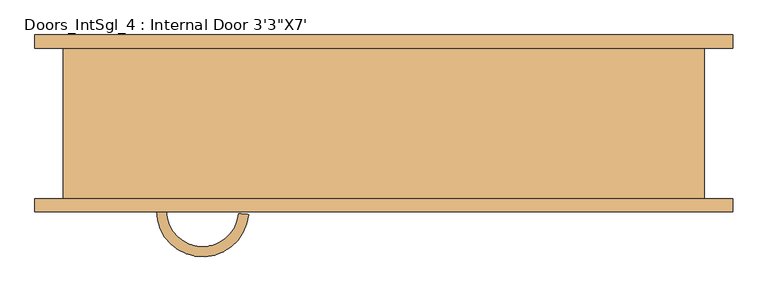
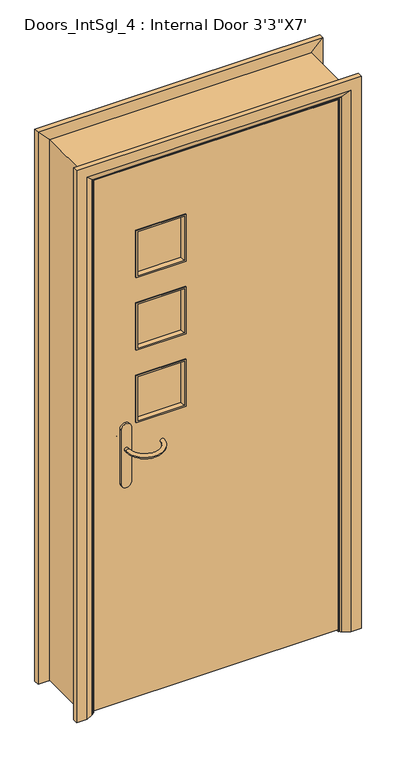
"""IFC4 building model written with IfcOpenShell, lengths in millimetres: door geometry."""

from ifc_helpers import new_model, si_unit, point, frame, frame_2d, origin, place, context, project, spatial, polyline, circle_curve, ellipse_curve, trimmed, segment, composite_curve, outline, extrude, faceted_brep, source, transform, mapped, element, save
from ifc_brep_helpers import plane_surface, cylinder_surface, revolved_surface, advanced_brep


def door_cca51ba5(model_context):
    return source(origin(), model_context, "Body", "SolidModel", [
        advanced_brep(
        [(-345.5, -68.3, 1000.0), (-330.5, -68.3, 1000.0), (-345.5, -58.3, 1000.0), (-330.5, -58.3, 1000.0), (-205.5986682, -52.1917759, 1000.0), (-220.5415886, -53.4991121, 1000.0)],
        [
            (0, 1, circle_curve(frame((-338.0, -68.3, 1000.0), z_axis=(0.0, -1.0, 0.0), x_axis=(1.0, 0.0, 0.0)), 7.5)),
            (1, 0, circle_curve(frame((-338.0, -68.3, 1000.0), z_axis=(0.0, -1.0, 0.0), x_axis=(1.0, 0.0, 0.0)), 7.5)),
            (0, 2),
            (2, 3, circle_curve(frame((-338.0, -58.3, 1000.0), z_axis=(0.0, -1.0, 0.0), x_axis=(1.0, 0.0, 0.0)), 7.5)),
            (3, 1),
            (3, 2, circle_curve(frame((-338.0, -58.3, 1000.0), z_axis=(0.0, -1.0, 0.0), x_axis=(1.0, 0.0, 0.0)), 7.5)),
            (4, 5, circle_curve(frame((-213.0701284, -52.845444, 1000.0), z_axis=(0.08715574274766678, -0.9961946980917448, 0.0), x_axis=(-0.9961946980917448, -0.08715574274766678, 0.0)), 7.5)),
            (5, 4, circle_curve(frame((-213.0701284, -52.845444, 1000.0), z_axis=(0.08715574274766678, -0.9961946980917448, 0.0), x_axis=(-0.9961946980917448, -0.08715574274766678, 0.0)), 7.5)),
            (5, 3, circle_curve(frame((-275.4159887, -58.3, 1000.0), z_axis=(0.0, 0.0, 1.0), x_axis=(-1.0, 0.0, 0.0)), 55.0840113)),
            (2, 4, circle_curve(frame((-275.4159887, -58.3, 1000.0), z_axis=(0.0, 0.0, -1.0), x_axis=(-1.0, 0.0, 0.0)), 70.0840113)),
        ],
        [
            plane_surface(frame((-338.0, -68.3, 1000.0), z_axis=(0.0, -1.0, 0.0), x_axis=(0.0, 0.0, 1.0))),
            cylinder_surface(frame((-338.0, -68.3, 1000.0), z_axis=(0.0, -1.0, 0.0), x_axis=(1.0, 0.0, 0.0)), 7.5),
            plane_surface(frame((-213.0701284, -52.845444, 1000.0), z_axis=(0.08715574274766678, -0.9961946980917448, 0.0), x_axis=(0.0, 0.0, 1.0))),
            revolved_surface(trimmed(ellipse_curve(frame((-338.0, -58.3, 1000.0), z_axis=(0.0, -1.0, 0.0), x_axis=(1.0, 0.0, 0.0)), 7.5, 7.5), [point((-345.5, -58.3, 1000.0))], [point((-330.5, -58.3, 1000.0))], True, "CARTESIAN"), (-275.4159887, -58.3, 1000.0), (0.0, 0.0, -1.0)),
            revolved_surface(trimmed(ellipse_curve(frame((-338.0, -58.3, 1000.0), z_axis=(0.0, -1.0, 0.0), x_axis=(1.0, 0.0, 0.0)), 7.5, 7.5), [point((-330.5, -58.3, 1000.0))], [point((-345.5, -58.3, 1000.0))], True, "CARTESIAN"), (-275.4159887, -58.3, 1000.0), (0.0, 0.0, -1.0)),
        ],
        [
            (0, [[1, 2]]),
            (1, [[-1, 3, 4, 5]]),
            (1, [[-2, -5, 6, -3]]),
            (2, [[7, 8]]),
            (3, [[9, -4, 10, -8]]),
            (4, [[-10, -6, -9, -7]]),
        ],
    ),
        extrude(outline(composite_curve([segment(trimmed(circle_curve(frame_2d((870.0, -338.0)), 20.0), [point((870.0, -358.0))], [point((870.0, -318.0))], False, "CARTESIAN"), True, "CONTINUOUS"), segment(polyline([(870.0, -318.0), (1080.0, -318.0)]), True, "CONTINUOUS"), segment(trimmed(circle_curve(frame_2d((1080.0, -338.0)), 20.0), [point((1080.0, -318.0))], [point((1080.0, -358.0))], False, "CARTESIAN"), True, "CONTINUOUS"), segment(polyline([(1080.0, -358.0), (870.0, -358.0)]), True, "CONTINUOUS")], self_intersect=False)), frame((0.0, -76.3, 0.0), z_axis=(0.0, 1.0, 0.0), x_axis=(0.0, 0.0, 1.0)), (0.0, 0.0, 1.0), 8.0),
        advanced_brep(
        [(-345.5, -122.3, 1000.0), (-330.5, -122.3, 1000.0), (-330.5, -132.3, 1000.0), (-345.5, -132.3, 1000.0), (-205.5986682, -138.4082241, 1000.0), (-220.5415886, -137.1008879, 1000.0)],
        [
            (0, 1, circle_curve(frame((-338.0, -122.3, 1000.0), z_axis=(0.0, 1.0, 0.0), x_axis=(1.0, 0.0, 0.0)), 7.5)),
            (1, 0, circle_curve(frame((-338.0, -122.3, 1000.0), z_axis=(0.0, 1.0, 0.0), x_axis=(1.0, 0.0, 0.0)), 7.5)),
            (1, 2),
            (2, 3, circle_curve(frame((-338.0, -132.3, 1000.0), z_axis=(0.0, 1.0, 0.0), x_axis=(1.0, 0.0, 0.0)), 7.5)),
            (3, 0),
            (3, 2, circle_curve(frame((-338.0, -132.3, 1000.0), z_axis=(0.0, 1.0, 0.0), x_axis=(1.0, 0.0, 0.0)), 7.5)),
            (4, 5, circle_curve(frame((-213.0701284, -137.754556, 1000.0), z_axis=(0.08715574274766356, 0.9961946980917451, 0.0), x_axis=(-0.9961946980917451, 0.08715574274766356, 0.0)), 7.5)),
            (5, 4, circle_curve(frame((-213.0701284, -137.754556, 1000.0), z_axis=(0.08715574274766356, 0.9961946980917451, 0.0), x_axis=(-0.9961946980917451, 0.08715574274766356, 0.0)), 7.5)),
            (4, 3, circle_curve(frame((-275.4159887, -132.3, 1000.0), z_axis=(0.0, 0.0, -1.0), x_axis=(-1.0, 0.0, 0.0)), 70.0840113)),
            (2, 5, circle_curve(frame((-275.4159887, -132.3, 1000.0), z_axis=(0.0, 0.0, 1.0), x_axis=(-1.0, 0.0, 0.0)), 55.0840113)),
        ],
        [
            plane_surface(frame((-338.0, -122.3, 1000.0), z_axis=(0.0, 1.0, 0.0), x_axis=(0.0, 0.0, 1.0))),
            cylinder_surface(frame((-338.0, -122.3, 1000.0), z_axis=(0.0, 1.0, 0.0), x_axis=(1.0, 0.0, 0.0)), 7.5),
            plane_surface(frame((-213.0701284, -137.754556, 1000.0), z_axis=(0.08715574274766356, 0.9961946980917451, 0.0), x_axis=(0.0, 0.0, 1.0))),
            revolved_surface(trimmed(ellipse_curve(frame((-338.0, -132.3, 1000.0), z_axis=(0.0, -1.0, 0.0), x_axis=(1.0, 0.0, 0.0)), 7.5, 7.5), [point((-345.5, -132.3, 1000.0))], [point((-330.5, -132.3, 1000.0))], True, "CARTESIAN"), (-275.4159887, -132.3, 1000.0), (0.0, 0.0, -1.0)),
            revolved_surface(trimmed(ellipse_curve(frame((-338.0, -132.3, 1000.0), z_axis=(0.0, -1.0, 0.0), x_axis=(1.0, 0.0, 0.0)), 7.5, 7.5), [point((-330.5, -132.3, 1000.0))], [point((-345.5, -132.3, 1000.0))], True, "CARTESIAN"), (-275.4159887, -132.3, 1000.0), (0.0, 0.0, -1.0)),
        ],
        [
            (0, [[1, 2]]),
            (1, [[3, 4, 5, -2]]),
            (1, [[-5, 6, -3, -1]]),
            (2, [[7, 8]]),
            (3, [[-7, 9, -4, 10]]),
            (4, [[-8, -10, -6, -9]]),
        ],
    ),
        extrude(outline(composite_curve([segment(trimmed(circle_curve(frame_2d((870.0, -338.0)), 20.0), [point((870.0, -358.0))], [point((870.0, -318.0))], False, "CARTESIAN"), True, "CONTINUOUS"), segment(polyline([(870.0, -318.0), (1080.0, -318.0)]), True, "CONTINUOUS"), segment(trimmed(circle_curve(frame_2d((1080.0, -338.0)), 20.0), [point((1080.0, -318.0))], [point((1080.0, -358.0))], False, "CARTESIAN"), True, "CONTINUOUS"), segment(polyline([(1080.0, -358.0), (870.0, -358.0)]), True, "CONTINUOUS")], self_intersect=False)), frame((0.0, -122.3, 0.0), z_axis=(0.0, 1.0, 0.0), x_axis=(0.0, 0.0, 1.0)), (0.0, 0.0, 1.0), 8.0),
        extrude(outline(polyline([(2091.6, -453.3), (8.0, -453.3), (8.0, 453.3), (2091.6, 453.3), (2091.6, -453.3)]), holes=[polyline([(1841.6, -113.3), (1656.6, -113.3), (1656.6, -298.3), (1841.6, -298.3), (1841.6, -113.3)]), polyline([(1086.6, -298.3), (1271.6, -298.3), (1271.6, -113.3), (1086.6, -113.3), (1086.6, -298.3)]), polyline([(1556.6, -113.3), (1371.6, -113.3), (1371.6, -298.3), (1556.6, -298.3), (1556.6, -113.3)])]), frame((0.0, -114.3, 0.0), z_axis=(0.0, 1.0, 0.0), x_axis=(0.0, 0.0, 1.0)), (0.0, 0.0, 1.0), 38.0),
        faceted_brep([(-455.3, -114.3, 0.0), (-487.3, -114.3, 0.0), (-487.3, 114.3, 0.0), (-455.3, 114.3, 0.0), (-455.3, 114.3, 2093.6), (-455.3, -114.3, 2093.6), (-487.3, 114.3, 2125.6), (-487.3, -114.3, 2125.6), (455.3, -114.3, 0.0), (455.3, 114.3, 0.0), (487.3, 114.3, 0.0), (487.3, -114.3, 0.0), (455.3, -114.3, 2093.6), (487.3, -114.3, 2125.6), (487.3, 114.3, 2125.6), (455.3, 114.3, 2093.6)], [[[0, 1, 2, 3]], [[3, 4, 5, 0]], [[2, 6, 4, 3]], [[1, 7, 6, 2]], [[0, 5, 7, 1]], [[8, 9, 10, 11]], [[12, 8, 11, 13]], [[13, 11, 10, 14]], [[14, 10, 9, 15]], [[15, 9, 8, 12]], [[4, 15, 12, 5]], [[6, 14, 15, 4]], [[7, 13, 14, 6]], [[5, 12, 13, 7]]]),
        advanced_brep(
        [(-530.3, 134.3, 0.0), (-490.3, 134.3, 0.0), (-464.3, 120.3, 0.0), (-460.3, 114.3, 0.0), (-530.3, 114.3, 0.0), (-530.3, 114.3, 2168.6), (-530.3, 134.3, 2168.6), (-460.3, 114.3, 2098.6), (-464.3, 120.3, 2102.6), (-490.3, 134.3, 2128.6), (530.3, 134.3, 0.0), (530.3, 114.3, 0.0), (460.3, 114.3, 0.0), (464.3, 120.3, 0.0), (490.3, 134.3, 0.0), (530.3, 134.3, 2168.6), (490.3, 134.3, 2128.6), (464.3, 120.3, 2102.6), (460.3, 114.3, 2098.6), (530.3, 114.3, 2168.6)],
        [
            (0, 1),
            (1, 2),
            (2, 3, circle_curve(frame((-468.3, 113.3, 0.0), z_axis=(0.0, 0.0, -1.0), x_axis=(-1.0, 0.0, 0.0)), 8.0622577)),
            (3, 4),
            (4, 0),
            (4, 5),
            (5, 6),
            (6, 0),
            (3, 7),
            (7, 5),
            (2, 8),
            (8, 7, ellipse_curve(frame((-468.3, 113.3, 2106.6), z_axis=(-0.7071067811865475, 0.0, -0.7071067811865475), x_axis=(0.7071067811865474, 0.0, -0.7071067811865476)), 11.4017543, 8.0622577)),
            (1, 9),
            (9, 8),
            (6, 9),
            (10, 11),
            (11, 12),
            (12, 13, circle_curve(frame((468.3, 113.3, 0.0), z_axis=(0.0, 0.0, -1.0), x_axis=(1.0, 0.0, 0.0)), 8.0622577)),
            (13, 14),
            (14, 10),
            (15, 10),
            (14, 16),
            (16, 15),
            (13, 17),
            (17, 16),
            (12, 18),
            (18, 17, ellipse_curve(frame((468.3, 113.3, 2106.6), z_axis=(0.7071067811865475, 0.0, -0.7071067811865475), x_axis=(0.7071067811865474, 0.0, 0.7071067811865476)), 11.4017543, 8.0622577)),
            (11, 19),
            (19, 18),
            (15, 19),
            (5, 19),
            (15, 6),
            (7, 18),
            (8, 17),
            (9, 16),
        ],
        [
            plane_surface(frame((-460.3, 187.1010989, 0.0), z_axis=(0.0, 0.0, -1.0), x_axis=(1.0, 0.0, 0.0))),
            plane_surface(frame((-530.3, 134.3, 0.0), z_axis=(-1.0, 0.0, 0.0), x_axis=(0.0, 0.0, 1.0))),
            plane_surface(frame((-530.3, 114.3, 0.0), z_axis=(0.0, -1.0, 0.0), x_axis=(0.0, 0.0, 1.0))),
            cylinder_surface(frame((-468.3, 113.3, 0.0), z_axis=(0.0, 0.0, -1.0), x_axis=(-1.0, 0.0, 0.0)), 8.0622577),
            plane_surface(frame((-464.3, 120.3, 0.0), z_axis=(0.4740998230350183, 0.8804710999221749, 0.0), x_axis=(0.0, 0.0, 1.0))),
            plane_surface(frame((-490.3, 134.3, 0.0), z_axis=(0.0, 1.0, 0.0), x_axis=(0.0, 0.0, 1.0))),
            plane_surface(frame((460.3, 187.1010989, 0.0), z_axis=(0.0, 0.0, -1.0), x_axis=(-1.0, 0.0, 0.0))),
            plane_surface(frame((490.3, 134.3, 2128.6), z_axis=(0.0, 1.0, 0.0), x_axis=(0.0, 0.0, -1.0))),
            plane_surface(frame((464.3, 120.3, 2102.6), z_axis=(-0.4740998230350183, 0.8804710999221749, 0.0), x_axis=(0.0, 0.0, -1.0))),
            cylinder_surface(frame((468.3, 113.3, 2098.6), z_axis=(0.0, 0.0, 1.0), x_axis=(1.0, 0.0, 0.0)), 8.0622577),
            plane_surface(frame((530.3, 114.3, 2168.6), z_axis=(0.0, -1.0, 0.0), x_axis=(0.0, 0.0, -1.0))),
            plane_surface(frame((530.3, 134.3, 2168.6), z_axis=(1.0, 0.0, 0.0), x_axis=(0.0, 0.0, -1.0))),
            plane_surface(frame((-530.3, 134.3, 2168.6), z_axis=(0.0, 0.0, 1.0), x_axis=(1.0, 0.0, 0.0))),
            plane_surface(frame((-530.3, 114.3, 2168.6), z_axis=(0.0, -1.0, 0.0), x_axis=(1.0, 0.0, 0.0))),
            cylinder_surface(frame((-460.3, 113.3, 2106.6), z_axis=(-1.0, 0.0, 0.0), x_axis=(0.0, 0.0, 1.0)), 8.0622577),
            plane_surface(frame((-464.3, 120.3, 2102.6), z_axis=(0.0, 0.8804710999221749, -0.4740998230350183), x_axis=(1.0, 0.0, 0.0))),
            plane_surface(frame((-490.3, 134.3, 2128.6), z_axis=(0.0, 1.0, 0.0), x_axis=(1.0, 0.0, 0.0))),
        ],
        [
            (0, [[1, 2, 3, 4, 5]]),
            (1, [[6, 7, 8, -5]]),
            (2, [[9, 10, -6, -4]]),
            (3, [[11, 12, -9, -3]]),
            (4, [[13, 14, -11, -2]]),
            (5, [[-8, 15, -13, -1]]),
            (6, [[16, 17, 18, 19, 20]]),
            (7, [[21, -20, 22, 23]]),
            (8, [[-22, -19, 24, 25]]),
            (9, [[-24, -18, 26, 27]]),
            (10, [[-26, -17, 28, 29]]),
            (11, [[-28, -16, -21, 30]]),
            (12, [[31, -30, 32, -7]]),
            (13, [[33, -29, -31, -10]]),
            (14, [[34, -27, -33, -12]]),
            (15, [[35, -25, -34, -14]]),
            (16, [[-32, -23, -35, -15]]),
        ],
    ),
        extrude(outline(polyline([(0.0, -436.3), (2074.6, -436.3), (2074.6, 436.3), (0.0, 436.3), (0.0, 455.3), (2093.6, 455.3), (2093.6, -455.3), (0.0, -455.3), (0.0, -436.3)])), frame((0.0, -74.3, 0.0), z_axis=(0.0, 1.0, 0.0), x_axis=(0.0, 0.0, 1.0)), (0.0, 0.0, 1.0), 32.0),
        advanced_brep(
        [(530.3, -134.3, 0.0), (490.3, -134.3, 0.0), (464.3, -120.3, 0.0), (460.3, -114.3, 0.0), (530.3, -114.3, 0.0), (530.3, -114.3, 2168.6), (530.3, -134.3, 2168.6), (460.3, -114.3, 2098.6), (-460.3, -114.3, 2098.6), (-460.3, -114.3, 0.0), (-530.3, -114.3, 0.0), (-530.3, -114.3, 2168.6), (464.3, -120.3, 2102.6), (490.3, -134.3, 2128.6), (-530.3, -134.3, 2168.6), (-530.3, -134.3, 0.0), (-490.3, -134.3, 0.0), (-490.3, -134.3, 2128.6), (-464.3, -120.3, 0.0), (-464.3, -120.3, 2102.6)],
        [
            (0, 1),
            (1, 2),
            (2, 3, circle_curve(frame((468.3, -113.3, 0.0), z_axis=(0.0, 0.0, -1.0), x_axis=(1.0, 0.0, 0.0)), 8.0622577)),
            (3, 4),
            (4, 0),
            (4, 5),
            (5, 6),
            (6, 0),
            (3, 7),
            (7, 8),
            (8, 9),
            (9, 10),
            (10, 11),
            (11, 5),
            (2, 12),
            (12, 7, ellipse_curve(frame((468.3, -113.3, 2106.6), z_axis=(0.7071067811865475, 0.0, -0.7071067811865475), x_axis=(-0.7071067811865474, 0.0, -0.7071067811865476)), 11.4017543, 8.0622577)),
            (1, 13),
            (13, 12),
            (6, 14),
            (14, 15),
            (15, 16),
            (16, 17),
            (17, 13),
            (10, 15),
            (14, 11),
            (9, 18, circle_curve(frame((-468.3, -113.3, 0.0), z_axis=(0.0, 0.0, -1.0), x_axis=(-1.0, 0.0, 0.0)), 8.0622577)),
            (18, 16),
            (19, 18),
            (8, 19, ellipse_curve(frame((-468.3, -113.3, 2106.6), z_axis=(-0.7071067811865475, 0.0, -0.7071067811865475), x_axis=(-0.7071067811865474, 0.0, 0.7071067811865476)), 11.4017543, 8.0622577)),
            (19, 17),
            (12, 19),
        ],
        [
            plane_surface(frame((460.3, -114.3, 0.0), z_axis=(0.0, 0.0, -1.0), x_axis=(0.0, 1.0, 0.0))),
            plane_surface(frame((530.3, -134.3, 0.0), z_axis=(1.0, 0.0, 0.0), x_axis=(0.0, 0.0, 1.0))),
            plane_surface(frame((530.3, -114.3, 0.0), z_axis=(0.0, 1.0, 0.0), x_axis=(0.0, 0.0, 1.0))),
            cylinder_surface(frame((468.3, -113.3, 0.0), z_axis=(0.0, 0.0, -1.0), x_axis=(1.0, 0.0, 0.0)), 8.0622577),
            plane_surface(frame((464.3, -120.3, 0.0), z_axis=(-0.4740998230350126, -0.8804710999221779, 0.0), x_axis=(0.0, 0.0, 1.0))),
            plane_surface(frame((490.3, -134.3, 0.0), z_axis=(0.0, -1.0, 0.0), x_axis=(0.0, 0.0, 1.0))),
            plane_surface(frame((-530.3, -134.3, 2168.6), z_axis=(-1.0, 0.0, 0.0), x_axis=(0.0, 0.0, -1.0))),
            plane_surface(frame((-460.3, -114.3, 0.0), z_axis=(0.0, 0.0, -1.0), x_axis=(0.0, 1.0, 0.0))),
            cylinder_surface(frame((-468.3, -113.3, 2098.6), z_axis=(0.0, 0.0, 1.0), x_axis=(-1.0, 0.0, 0.0)), 8.0622577),
            plane_surface(frame((-464.3, -120.3, 2102.6), z_axis=(0.4740998230350183, -0.8804710999221749, 0.0), x_axis=(0.0, 0.0, -1.0))),
            plane_surface(frame((530.3, -134.3, 2168.6), z_axis=(0.0, 0.0, 1.0), x_axis=(-1.0, 0.0, 0.0))),
            cylinder_surface(frame((460.3, -113.3, 2106.6), z_axis=(1.0, 0.0, 0.0), x_axis=(0.0, 0.0, 1.0)), 8.0622577),
            plane_surface(frame((464.3, -120.3, 2102.6), z_axis=(0.0, -0.8804710999221763, -0.4740998230350154), x_axis=(-1.0, 0.0, 0.0))),
        ],
        [
            (0, [[1, 2, 3, 4, 5]]),
            (1, [[6, 7, 8, -5]]),
            (2, [[9, 10, 11, 12, 13, 14, -6, -4]]),
            (3, [[15, 16, -9, -3]]),
            (4, [[17, 18, -15, -2]]),
            (5, [[-8, 19, 20, 21, 22, 23, -17, -1]]),
            (6, [[-13, 24, -20, 25]]),
            (7, [[-24, -12, 26, 27, -21]]),
            (8, [[28, -26, -11, 29]]),
            (9, [[-22, -27, -28, 30]]),
            (10, [[-14, -25, -19, -7]]),
            (11, [[31, -29, -10, -16]]),
            (12, [[-23, -30, -31, -18]]),
        ],
    ),
        faceted_brep([(-113.3, -117.3, 1841.6), (-113.3, -117.3, 1656.6), (-113.3, -104.3, 1656.6), (-113.3, -104.3, 1841.6), (-125.3, -104.3, 1829.6), (-125.3, -104.3, 1668.6), (-119.3, -117.3, 1662.6), (-119.3, -117.3, 1835.6), (-298.3, -117.3, 1656.6), (-298.3, -104.3, 1656.6), (-286.3, -104.3, 1668.6), (-292.3, -117.3, 1662.6), (-298.3, -117.3, 1841.6), (-298.3, -104.3, 1841.6), (-286.3, -104.3, 1829.6), (-292.3, -117.3, 1835.6)], [[[0, 1, 2, 3]], [[4, 5, 6, 7]], [[1, 8, 9, 2]], [[5, 10, 11, 6]], [[8, 12, 13, 9]], [[10, 14, 15, 11]], [[3, 2, 9, 13], [5, 4, 14, 10]], [[12, 0, 3, 13]], [[1, 0, 12, 8], [7, 6, 11, 15]], [[14, 4, 7, 15]]]),
        faceted_brep([(-119.3, -73.3, 1835.6), (-119.3, -73.3, 1662.6), (-125.3, -86.3, 1668.6), (-125.3, -86.3, 1829.6), (-113.3, -86.3, 1841.6), (-113.3, -86.3, 1656.6), (-113.3, -73.3, 1656.6), (-113.3, -73.3, 1841.6), (-292.3, -73.3, 1662.6), (-286.3, -86.3, 1668.6), (-298.3, -86.3, 1656.6), (-298.3, -73.3, 1656.6), (-292.3, -73.3, 1835.6), (-286.3, -86.3, 1829.6), (-298.3, -86.3, 1841.6), (-298.3, -73.3, 1841.6)], [[[0, 1, 2, 3]], [[4, 5, 6, 7]], [[1, 8, 9, 2]], [[5, 10, 11, 6]], [[8, 12, 13, 9]], [[10, 14, 15, 11]], [[12, 0, 3, 13]], [[7, 6, 11, 15], [1, 0, 12, 8]], [[14, 4, 7, 15]], [[5, 4, 14, 10], [3, 2, 9, 13]]]),
        extrude(outline(polyline([(-298.3, -104.3), (-298.3, -86.3), (-113.3, -86.3), (-113.3, -104.3), (-298.3, -104.3)])), frame((0.0, 0.0, 1656.6), z_axis=(0.0, 0.0, 1.0), x_axis=(1.0, 0.0, 0.0)), (0.0, 0.0, 1.0), 185.0),
        extrude(outline(polyline([(-298.3, -104.3), (-298.3, -86.3), (-113.3, -86.3), (-113.3, -104.3), (-298.3, -104.3)])), frame((0.0, 0.0, 1086.6), z_axis=(0.0, 0.0, 1.0), x_axis=(1.0, 0.0, 0.0)), (0.0, 0.0, 1.0), 185.0),
        extrude(outline(polyline([(-298.3, -104.3), (-298.3, -86.3), (-113.3, -86.3), (-113.3, -104.3), (-298.3, -104.3)])), frame((0.0, 0.0, 1371.6), z_axis=(0.0, 0.0, 1.0), x_axis=(1.0, 0.0, 0.0)), (0.0, 0.0, 1.0), 185.0),
        faceted_brep([(-298.3, -117.3, 1371.6), (-298.3, -117.3, 1556.6), (-298.3, -104.3, 1556.6), (-298.3, -104.3, 1371.6), (-286.3, -104.3, 1383.6), (-286.3, -104.3, 1544.6), (-292.3, -117.3, 1550.6), (-292.3, -117.3, 1377.6), (-113.3, -117.3, 1556.6), (-113.3, -104.3, 1556.6), (-125.3, -104.3, 1544.6), (-119.3, -117.3, 1550.6), (-113.3, -117.3, 1371.6), (-113.3, -104.3, 1371.6), (-125.3, -104.3, 1383.6), (-119.3, -117.3, 1377.6)], [[[0, 1, 2, 3]], [[4, 5, 6, 7]], [[1, 8, 9, 2]], [[5, 10, 11, 6]], [[8, 12, 13, 9]], [[10, 14, 15, 11]], [[3, 2, 9, 13], [5, 4, 14, 10]], [[12, 0, 3, 13]], [[1, 0, 12, 8], [7, 6, 11, 15]], [[14, 4, 7, 15]]]),
        faceted_brep([(-298.3, -117.3, 1086.6), (-298.3, -117.3, 1271.6), (-298.3, -104.3, 1271.6), (-298.3, -104.3, 1086.6), (-286.3, -104.3, 1098.6), (-286.3, -104.3, 1259.6), (-292.3, -117.3, 1265.6), (-292.3, -117.3, 1092.6), (-113.3, -117.3, 1271.6), (-113.3, -104.3, 1271.6), (-125.3, -104.3, 1259.6), (-119.3, -117.3, 1265.6), (-113.3, -117.3, 1086.6), (-113.3, -104.3, 1086.6), (-125.3, -104.3, 1098.6), (-119.3, -117.3, 1092.6)], [[[0, 1, 2, 3]], [[4, 5, 6, 7]], [[1, 8, 9, 2]], [[5, 10, 11, 6]], [[8, 12, 13, 9]], [[10, 14, 15, 11]], [[3, 2, 9, 13], [5, 4, 14, 10]], [[12, 0, 3, 13]], [[1, 0, 12, 8], [7, 6, 11, 15]], [[14, 4, 7, 15]]]),
        faceted_brep([(-113.3, -73.3, 1371.6), (-113.3, -73.3, 1556.6), (-113.3, -86.3, 1556.6), (-113.3, -86.3, 1371.6), (-125.3, -86.3, 1383.6), (-125.3, -86.3, 1544.6), (-119.3, -73.3, 1550.6), (-119.3, -73.3, 1377.6), (-298.3, -73.3, 1556.6), (-298.3, -86.3, 1556.6), (-286.3, -86.3, 1544.6), (-292.3, -73.3, 1550.6), (-298.3, -73.3, 1371.6), (-298.3, -86.3, 1371.6), (-286.3, -86.3, 1383.6), (-292.3, -73.3, 1377.6)], [[[0, 1, 2, 3]], [[4, 5, 6, 7]], [[1, 8, 9, 2]], [[5, 10, 11, 6]], [[8, 12, 13, 9]], [[10, 14, 15, 11]], [[3, 2, 9, 13], [5, 4, 14, 10]], [[12, 0, 3, 13]], [[1, 0, 12, 8], [7, 6, 11, 15]], [[14, 4, 7, 15]]]),
        faceted_brep([(-113.3, -73.3, 1086.6), (-113.3, -73.3, 1271.6), (-113.3, -86.3, 1271.6), (-113.3, -86.3, 1086.6), (-125.3, -86.3, 1098.6), (-125.3, -86.3, 1259.6), (-119.3, -73.3, 1265.6), (-119.3, -73.3, 1092.6), (-298.3, -73.3, 1271.6), (-298.3, -86.3, 1271.6), (-286.3, -86.3, 1259.6), (-292.3, -73.3, 1265.6), (-298.3, -73.3, 1086.6), (-298.3, -86.3, 1086.6), (-286.3, -86.3, 1098.6), (-292.3, -73.3, 1092.6)], [[[0, 1, 2, 3]], [[4, 5, 6, 7]], [[1, 8, 9, 2]], [[5, 10, 11, 6]], [[8, 12, 13, 9]], [[10, 14, 15, 11]], [[3, 2, 9, 13], [5, 4, 14, 10]], [[12, 0, 3, 13]], [[1, 0, 12, 8], [7, 6, 11, 15]], [[14, 4, 7, 15]]]),
    ])


if __name__ == "__main__":
    model = new_model("IFC4")
    model_context = context("Model", 3, world=origin())
    ifc_project = project(units=[si_unit("LENGTHUNIT", "METRE", prefix="MILLI")], contexts=[model_context])
    site = spatial("IfcSite", under=ifc_project)
    building = spatial("IfcBuilding", under=site)
    placement = place(None, origin())
    door_shape = door_cca51ba5(model_context)
    element("IfcDoor", 1, ObjectType="Doors_IntSgl_4 : Internal Door 3'3\"X7'", at=placement, inside=building, context=model_context, shape_type="MappedRepresentation", body=[
        mapped(door_shape, transform((0.0, 0.0, 0.0), x_axis=(1.0, 0.0, 0.0), y_axis=(0.0, 1.0, 0.0), z_axis=(0.0, 0.0, 1.0))),
    ])
    save(model, "model.ifc")

# Revit data of these elements
# Type "Doors_IntSgl_4 : Internal Door 3'3\"X7'"
#   Type Mark = "13"
#   Type Comments = "Internal Single"
#   Operation = "SingleSwingRight"
#   Construction Type Id = "SGL"
#   Manufacturer = "Revit"
#   Keynote = "L20"
#   Description = "Internal Single Door"
#   Analytic Construction = "Large single-glazed windows"
#   Visual Light Transmittance = 0.9
#   VisionPanel Width = 0' - 7.28346"
#   VisionPanel Depth = 0' - 7.28346"
#   UnderCut = 0' - 0.31496"
#   Tolerance = 0' - 0.07874"
#   Thickness = 0' - 1.49606"
#   Structural Tolerance = 0' - 0.31496"
#   StopDepth = 0' - 1.25984"
#   Stop Thickness = 0' - 0.74803"
#   Stile Shutting = 0' - 6.10236"
#   Stile Top Rail = 0' - 9.84252"
#   Stile Intermediate/Frieze = 0' - 3.93701"
#   Solar Heat Gain Coefficient = 0.86
#   Rough Width = 3' - 3"
#   Rough Height = 7' - 0"
#   Heat Transfer Coefficient (U) = 0.979472 BTU/(h·ft²·°F)
#   Handle Z Distance = 3' - 3.37008"
#   Handle X Distance = 0' - 2.95276"
#   Handle Length = 1' - 1.77953"
#   Frame Thickness = 0' - 1.25984"
#   Door Panel Width = 2' - 11.69291"
#   Door Panel Thickness = 0' - 1.49606"
#   Door Panel Offset = 0' - 0"
#   Height = 7' - 0"
#   Width = 3' - 3"
#   Door Panel Height = 6' - 10.0315"
#   Architrave Setback = 0' - 0.19685"
#   Vis - Ironmongery = yes
#   Define Thermal Properties by = 1
#   Material Ironmongery = Door - Handle
#   Material Glass = Door - Glazing
#   Material Frame = Door - Frame/Mullion
#   Material Door = Door - Panel
#   Material Beading = Door - Panel
#   Material Architrave = Door - Architrave
#   Handle Style = element 386699
#   Function = (empty or 0)
#   Wall Closure = (empty or 0)
# Element 1 (IfcDoor, "Doors_IntSgl_4 : Internal Door 3'3\"X7'")
#   Materials on its faces: "Door - Panel", "Door - Architrave", "Door - Handle", "Door - Frame/Mullion", "Door - Glazing"
# Materials
#   "Door - Handle": colour RGB 247 247 247, transparency 0
#   "Door - Glazing": colour RGB 0 0 255, transparency 0.75
#   "Door - Frame/Mullion": class "Wood", colour RGB 212 179 113, transparency 0
#   "Door - Panel": class "Wood", colour RGB 210 159 95, transparency 0, Cost = 0
#   "Door - Architrave": class "Wood", colour RGB 212 179 113, transparency 0
